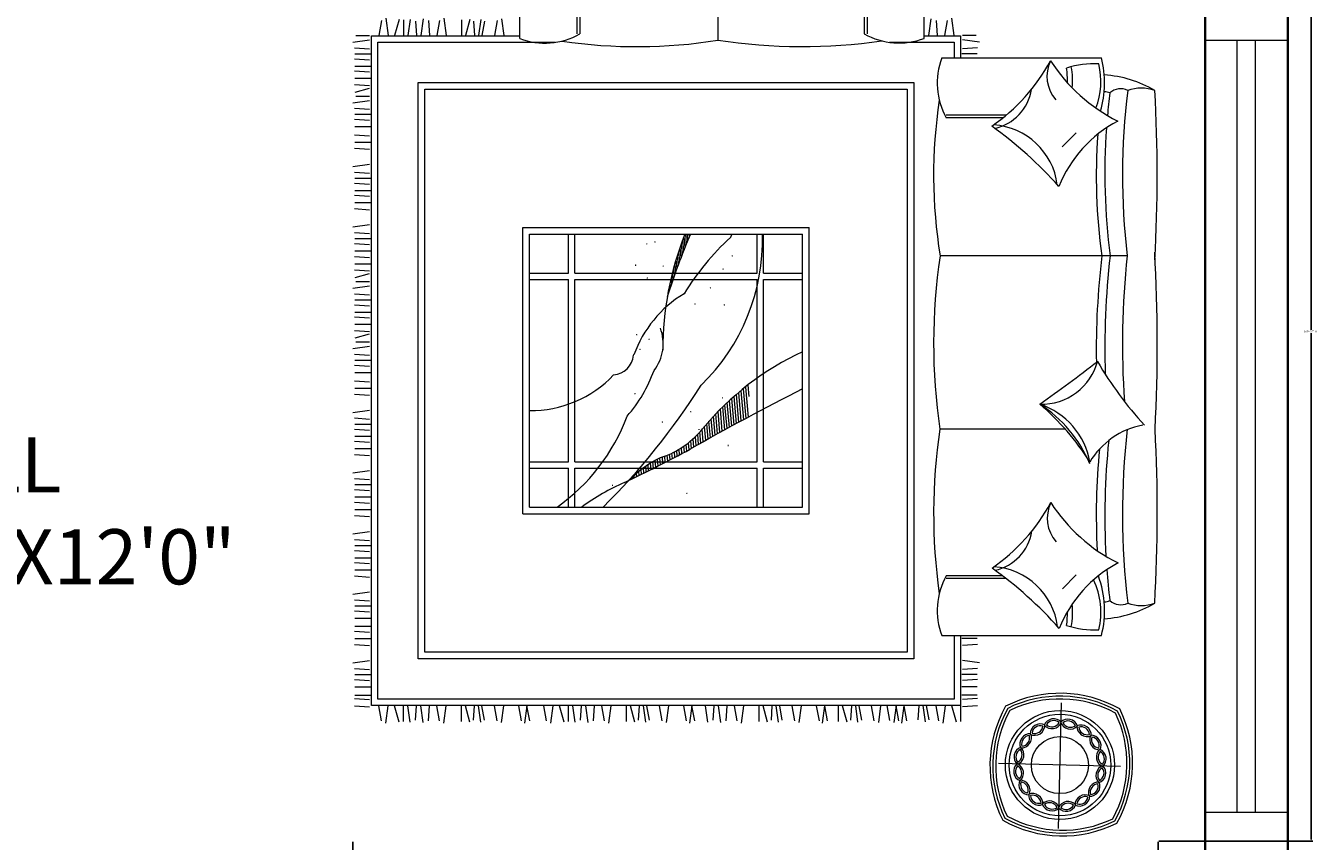
# Model space of a CAD drawing. Units: inches. Extents: x 1602 to 2642, y 1463 to 2270.
# Tile 3 of 5: x 1854 to 1995, y 1763 to 1851. Entities that reach past the tile are written whole.
import ezdxf

# ---------------------------------------------------------------- set-up
doc = ezdxf.new("R2010")
doc.units = ezdxf.units.IN
for name, color, linetype, lineweight in [('A-ANNO-DIMS', 2, 'Continuous', 18), ('A-AREA-IDEN', 7, 'Continuous', 18), ('A-FURN', 8, 'Continuous', 13), ('A-GLAZ', 4, 'Continuous', 18), ('A-WALL', 7, 'Continuous', 35)]:
    doc.layers.add(name, color=color, linetype=linetype, lineweight=lineweight)
doc.styles.get("Standard").update_dxf_attribs({"font": 'arial.ttf'})
doc.dimstyles.get("Standard").update_dxf_attribs({"dimtxt": 0.18, "dimasz": 0.18, "dimexe": 0.18, "dimexo": 0.0625, "dimgap": 0.09, "dimtad": 0, "dimtih": 1, "dimtoh": 1, "dimdec": 4, "dimzin": 0, "dimdsep": 46, "dimtxsty": 'Standard', "dimcen": 0.09, "dimadec": 0, "dimazin": 0, "dimtfac": 1, "dimtdec": 4, "dimtofl": 0, "dimtmove": 0, "dimatfit": 3, "dimfxl": 1, "dimtolj": 1, "dimtzin": 0, "dimarcsym": 0})

# ---------------------------------------------------------------- blocks, each defined once
blk = doc.blocks.new('A$C25EC1EFB')
h = blk.add_hatch()
h.set_pattern_fill('ANSI31', color=256, scale=2.508, angle=580, style=0)
h.set_pattern_definition([(94.99999999999984, (2801.512250582819, 4289.79602251789), (7.93259876143476, 0.6940124639253284), [])])
edge = h.paths.add_edge_path()
edge.add_ellipse((4084.490467177063, -2815.580363917667), major_axis=(-3872.16408689083, 3872.16408689083), ratio=0.9999999999995552, start_angle=340.89961915580596, end_angle=343.15488567038426, ccw=False)
edge.add_ellipse((1486.624568246823, 2293.159848771007), major_axis=(-194.6618757392838, 194.6618757392838), ratio=0.9999999999999246, start_angle=154.9056197196584, end_angle=183.4247301497222, ccw=False)
edge.add_ellipse((1687.117678346121, 1762.501521206774), major_axis=(-206.4950185728816, 206.4950185728816), ratio=0.999999999999898, start_angle=-23.5559095241906, end_angle=5.886608761987814)
edge.add_ellipse((823.8605303866296, 2467.162105106873), major_axis=(-581.4647167234576, 581.4647167234575), ratio=0.9999999999998493, start_angle=171.3363574034995, end_angle=185.7365630084011, ccw=False)
edge.add_line((1311.102457978037, 1804.744006331188), (1311.102457978037, 1908.515397835807))
edge.add_ellipse((-1407.416444189095, 7084.924681207201), major_axis=(4134.341428234145, 4134.341428234145), ratio=0.9999999999998351, start_angle=252.7073165240117, end_angle=254.8255249662156)
for p, q in [((317.5955949916479, 3231.219981357114), (307.6667150012017, 2827.177484563647)), ((117.9581545735291, 3031.926905659195), (509.944476949613, 3022.294292298837)), ((631.3901738150179, 2887.027849165279), (631.3901738150179, 2837.065101766894)), ((645.0795442243489, 2888.982161353262), (659.578070331745, 2837.065101766894)), ((688.1038474819233, 2892.890785729214), (680.5546081906668, 2837.065101766894)), ((701.7933985184081, 2885.073657987355), (710.5281339450539, 2837.065101766894)), ((732.7198837349368, 2882.204286455359), (741.09904921226, 2836.15004242288)), ((744.6795541957126, 2888.067102009248), (751.895255557758, 2836.15004242288)), ((767.9214057730514, 2882.204286455359), (764.7430494098026, 2836.15004242288)), ((804.5489009072134, 2885.073657987355), (813.2836363338665, 2837.065101766894)), ((820.5056566457297, 2892.890785729214), (812.9564173544732, 2837.065101766894)), ((830.489018271599, 2885.073657987355), (839.2237536982593, 2837.065101766894)), ((844.7281230778335, 2890.021414197218), (837.443163044978, 2836.15004242288)), ((858.8260332672307, 2884.158598643342), (867.5607686938984, 2836.15004242288)), ((894.9755861610774, 2890.936473541231), (887.690626128222, 2837.065101766894)), ((909.0734963504747, 2885.073657987355), (917.8082317771423, 2837.065101766894)), ((949.507840107568, 2883.119345799372), (957.8870055848911, 2837.065101766894)), ((961.4675105683438, 2888.982161353262), (968.683211930389, 2837.065101766894)), ((984.7093621456823, 2883.119345799372), (981.5310057824335, 2837.065101766894)), ((996.6690326064581, 2888.982161353262), (1011.167558713861, 2837.065101766894)), ((1023.822365107089, 2887.027849165279), (1023.822365107096, 2837.065101766894)), ((1059.561252837937, 2885.073657987355), (1068.29598826459, 2837.065101766894)), ((1075.518008576453, 2892.890785729214), (1067.968769285196, 2837.065101766894)), ((1085.501370202322, 2885.073657987355), (1094.236105628983, 2837.065101766894)), ((1149.987938091801, 2890.936473541231), (1142.702978058945, 2837.065101766894)), ((1164.085848281198, 2885.073657987355), (1172.820583707866, 2837.065101766894)), ((1204.520192038291, 2883.119345799372), (1212.899357515614, 2837.065101766894)), ((1216.479862499067, 2888.982161353262), (1223.695563861112, 2837.065101766894)), ((1239.721714076406, 2883.119345799372), (1236.543357713157, 2837.065101766894)), ((1251.681384537181, 2888.982161353262), (1266.179910644585, 2837.065101766894)), ((1278.834717037813, 2887.027849165279), (1278.83471703782, 2837.065101766894)), ((1335.548390704718, 2892.890785729214), (1327.999151413454, 2837.065101766894)), ((1349.237941741217, 2885.073657987355), (1357.972677167871, 2837.065101766894)), ((1384.439463779332, 2885.073657987355), (1381.126233840167, 2837.065101766894)), ((1402.040315111962, 2890.936473541231), (1409.52763688603, 2837.065101766894)), ((1426.2526619992, 2883.119345799372), (1423.074305635951, 2837.065101766894)), ((1443.853513331845, 2888.982161353262), (1451.069214693891, 2837.065101766894)), ((1485.909894853563, 2885.073657987355), (1494.644630280216, 2837.065101766894)), ((1501.866650592079, 2892.890785729214), (1494.317411300822, 2837.065101766894)), ((1511.850012217948, 2885.073657987355), (1520.584747644609, 2837.065101766894)), ((1576.336580107427, 2890.936473541231), (1569.051620074571, 2837.065101766894)), ((1590.434490296824, 2885.073657987355), (1599.169225723492, 2837.065101766894)), ((1630.868834053917, 2883.119345799372), (1639.247999531241, 2837.065101766894)), ((1642.828504514693, 2888.982161353262), (1650.044205876738, 2837.065101766894)), ((1666.070356092031, 2883.119345799372), (1662.891999728783, 2837.065101766894)), ((1678.030026552807, 2888.982161353262), (1692.528552660211, 2837.065101766894)), ((1705.183359053439, 2887.027849165279), (1705.183359053446, 2837.065101766894)), ((1761.897032720344, 2892.890785729214), (1754.34779342908, 2837.065101766894)), ((1775.586583756843, 2885.073657987355), (1784.321319183496, 2837.065101766894)), ((1810.788105794958, 2885.073657987355), (1807.474875855793, 2837.065101766894)), ((1828.388957127588, 2890.936473541231), (1835.876278901656, 2837.065101766894)), ((1852.601304014826, 2883.119345799372), (1849.422947651578, 2837.065101766894)), ((1870.202155347471, 2888.982161353262), (1877.417856709517, 2837.065101766894)), ((1891.714306976255, 2887.027849165279), (1891.714306976255, 2837.065101766894)), ((1905.403677385586, 2888.982161353262), (1919.902203492982, 2837.065101766894)), ((1948.427980643159, 2892.890785729214), (1940.878741351902, 2837.065101766894)), ((1962.117531679643, 2885.073657987355), (1970.852267106289, 2837.065101766894)), ((2015.857572578178, 2885.073657987355), (2024.592308004831, 2837.065101766894)), ((2031.814328316694, 2892.890785729214), (2024.265089025437, 2837.065101766894)), ((2041.797689942563, 2885.073657987355), (2050.532425369223, 2837.065101766894)), ((2106.284257832041, 2890.936473541231), (2098.999297799186, 2837.065101766894)), ((2120.382168021439, 2885.073657987355), (2129.116903448107, 2837.065101766894)), ((2160.816511778532, 2883.119345799372), (2169.195677255855, 2837.065101766894)), ((2172.776182239308, 2888.982161353262), (2179.991883601353, 2837.065101766894)), ((2196.018033816647, 2883.119345799372), (2192.839677453398, 2837.065101766894)), ((2207.977704277422, 2888.982161353262), (2222.476230384826, 2837.065101766894)), ((2235.131036778053, 2887.027849165279), (2235.131036778061, 2837.065101766894)), ((2291.844710444959, 2892.890785729214), (2284.295471153695, 2837.065101766894)), ((2305.534261481458, 2885.073657987355), (2314.268996908111, 2837.065101766894)), ((2340.735783519573, 2885.073657987355), (2337.422553580407, 2837.065101766894)), ((2358.336634852203, 2890.936473541231), (2365.823956626271, 2837.065101766894)), ((2382.548981739441, 2883.119345799372), (2379.370625376192, 2837.065101766894)), ((2400.149833072086, 2888.982161353262), (2407.365534434132, 2837.065101766894)), ((2421.66198470087, 2887.027849165279), (2421.66198470087, 2837.065101766894)), ((2435.351355110201, 2888.982161353262), (2449.849881217597, 2837.065101766894)), ((2478.375658367775, 2892.890785729214), (2470.826419076519, 2837.065101766894)), ((2492.06520940426, 2885.073657987355), (2500.799944830906, 2837.065101766894)), ((577.4890519529235, 2836.936244475415), (625.4976081733639, 2840.249474414588)), ((631.7592766263715, 2611.384835378944), (631.7592766263642, 2836.15004242288)), ((631.7592766263642, 2836.15004242288), (2524.304554552116, 2836.15004242288)), ((2524.304554552116, 2836.15004242288), (2524.304554552116, 684.1140680284224)), ((2578.574779225565, 2836.936244475415), (2530.566223005124, 2840.249474414588)), ((577.4890519529235, 2813.194849922737), (625.4976081733639, 2816.50807986191)), ((578.4283959861222, 2802.710657647047), (628.3911433845077, 2802.710657647047)), ((652.6592766263728, 2611.384835378944), (652.6592766263728, 2815.250042422886)), ((652.6592766263728, 2815.250042422886), (2503.404554552123, 2815.250042422886)), ((2503.404554552123, 2815.250042422886), (2503.404554552123, 705.0140680284312)), ((2577.635435192373, 2802.710657647047), (2527.672687793987, 2802.710657647047)), ((2578.574779225565, 2813.194849922737), (2530.566223005124, 2816.508079861895)), ((577.4890519529235, 2752.144911700663), (625.4976081733639, 2755.458141639836)), ((578.4283959861222, 2775.577635301154), (628.3911433845077, 2775.577635301154)), ((2577.635435192373, 2775.577635301154), (2527.672687793987, 2775.577635301154)), ((2578.574779225565, 2752.144911700663), (2530.566223005124, 2755.458141639836)), ((571.6262363990336, 2699.054774001932), (625.4976081733639, 2691.56745222785)), ((577.4890519529235, 2716.655625334541), (625.4976081733639, 2719.968855273714)), ((578.4283959861222, 2735.993497111231), (628.3911433845077, 2735.993497111231)), ((2577.635435192373, 2735.993497111231), (2527.672687793987, 2735.993497111231)), ((2578.574779225565, 2716.655625334541), (2530.566223005124, 2719.968855273714)), ((2584.437594779462, 2699.054774001932), (2530.566223005124, 2691.56745222785)), ((782.2392766263674, 834.5940680284328), (782.2392766263674, 2685.670042422884)), ((782.2392766263674, 2685.670042422884), (2373.824554552121, 2685.670042422884)), ((803.1392766263689, 855.4940680284271), (803.1392766263689, 2664.77004242289)), ((803.1392766263689, 2664.77004242289), (2352.924554552119, 2664.770042422875)), ((2352.924554552119, 2664.770042422875), (2352.924554552119, 855.4940680284271)), ((2373.824554552121, 2685.670042422884), (2373.824554552121, 834.5940680284328)), ((577.4890519529235, 2640.217478394574), (625.4976081733639, 2643.530708333732)), ((578.4283959861222, 2620.426176498651), (628.3911433845077, 2620.426176498651)), ((2577.635435192373, 2620.426176498651), (2527.672687793987, 2620.426176498651)), ((2578.574779225565, 2640.217478394574), (2530.566223005124, 2643.530708333732)), ((692.3034891433799, 2611.384835378944), (179.5334957905306, 2611.384835378958)), ((2577.635435192373, 2581.514517398078), (2527.672687793987, 2581.514517398078)), ((2578.574779225565, 2596.993452898176), (2530.566223005124, 2600.306682837334)), ((2577.635435192373, 2555.119914909323), (2527.672687793987, 2555.119914909323)), ((2578.574779225565, 2531.687191308833), (2530.566223005124, 2535.000421248005)), ((2577.635435192373, 2515.5357767194), (2527.672687793987, 2515.5357767194)), ((2578.574779225565, 2496.19790494271), (2530.566223005124, 2499.511134881883)), ((260.1263754639749, 2416.008756119314), (304.7479648114258, 2460.672138615999)), ((2584.437594779462, 2478.597053610102), (2530.566223005124, 2471.109731836019)), ((485.7932158359489, 2428.108270674471), (677.7791130337154, 2428.108270674471)), ((497.6695522999961, 2418.947027564289), (677.7791130337154, 2418.947027564289)), ((2578.574779225565, 2419.759758002729), (2530.566223005124, 2423.072987941902)), ((2577.635435192373, 2399.968456106821), (2527.672687793987, 2399.968456106821)), ((2578.574779225565, 2376.535732506331), (2530.566223005124, 2379.848962445518)), ((2577.635435192373, 2361.056797006248), (2527.672687793987, 2361.056797006248)), ((2578.574779225565, 2337.624073405757), (2530.566223005124, 2340.937303344916)), ((2577.635435192373, 2321.472658816325), (2527.672687793987, 2321.472658816325)), ((2578.574779225565, 2302.134787039635), (2530.566223005124, 2305.448016978807)), ((2584.437594779462, 2284.533935707012), (2530.566223005124, 2277.046613932944)), ((1118.231915589249, 2219.932055225661), (1118.231915589242, 1300.332055225655)), ((2037.831915589246, 2219.932055225647), (1118.231915589249, 2219.932055225661)), ((2037.831915589246, 2219.932055225647), (2037.831915589246, 1300.332055225655)), ((2577.635435192373, 2205.905338203745), (2527.672687793987, 2205.905338203745)), ((2578.574779225565, 2225.696640099654), (2530.566223005124, 2229.009870038812)), ((2016.931915589244, 2199.032055225638), (1139.131915589243, 2199.032055225638)), ((1139.131915589243, 2199.032055225638), (1139.131915589243, 1321.232055225664)), ((1264.531915589245, 2199.032055225638), (1264.531915589245, 2073.63205522563)), ((1285.431915589246, 2199.032055225638), (1285.431915589246, 2073.63205522563)), ((1870.631915589243, 2199.032055225638), (1870.631915589243, 2073.632055225644)), ((1891.531915589245, 2199.032055225638), (1891.531915589245, 2073.632055225644)), ((2016.931915589244, 2199.032055225638), (2016.931915589244, 1321.23205522565)), ((2577.635435192373, 2165.079528967945), (2527.672687793987, 2165.079528967945)), ((2578.574779225565, 2182.472614603256), (2530.566223005124, 2185.785844542428)), ((2577.635435192373, 2125.495390778036), (2527.672687793987, 2125.495390778036)), ((2578.574779225565, 2141.646805367455), (2530.566223005124, 2144.960035306627)), ((2578.574779225565, 2106.157519001346), (2530.566223005124, 2109.470748940505)), ((2584.437594779462, 2088.556667668723), (2530.566223005124, 2081.069345894641)), ((1264.531915589245, 2073.63205522563), (1139.131915589243, 2073.632055225644)), ((1264.531915589245, 2052.732055225635), (1139.131915589243, 2052.732055225664)), ((1264.531915589245, 2052.732055225635), (1264.531915589245, 1467.532055225652)), ((1870.631915589243, 2073.632055225644), (1285.431915589246, 2073.63205522563)), ((1870.631915589243, 2052.73205522565), (1285.431915589246, 2052.732055225635)), ((1285.431915589246, 2052.732055225635), (1285.431915589246, 1467.532055225652)), ((1870.631915589243, 2052.73205522565), (1870.631915589243, 1467.532055225652)), ((2016.931915589244, 2073.632055225658), (1891.531915589245, 2073.632055225644)), ((1891.531915589245, 2052.73205522565), (1891.531915589245, 1467.532055225652)), ((2016.931915589244, 2052.73205522565), (1891.531915589245, 2052.73205522565)), ((2577.635435192373, 2009.928070165443), (2527.672687793987, 2009.928070165443)), ((2578.574779225565, 2029.71937206135), (2530.566223005124, 2033.032602000523)), ((2577.635435192373, 1971.016411064869), (2527.672687793987, 1971.016411064869)), ((2578.574779225565, 1986.495346564967), (2530.566223005124, 1989.80857650414)), ((295.215244063229, 1948.444262769866), (698.1955948366831, 1948.444262769866)), ((2577.635435192373, 1931.432272874946), (2527.672687793987, 1931.432272874946)), ((2578.574779225565, 1947.583687464379), (2530.566223005124, 1950.896917403552)), ((2578.574779225565, 1912.094401098256), (2530.566223005124, 1915.407631037429)), ((2584.437594779454, 1894.493549765633), (2530.566223005124, 1887.006227991565)), ((2578.574779225565, 1835.656254158275), (2530.566223005124, 1838.969484097433)), ((2577.635435192373, 1815.864952262367), (2527.672687793987, 1815.864952262367)), ((2578.574779225565, 1792.432228661877), (2530.566223005124, 1795.74545860105)), ((2577.635435192373, 1765.828830553167), (2527.672687793987, 1765.828830553167)), ((2578.574779225565, 1742.396106952677), (2530.566223005124, 1745.70933689185)), ((2577.635435192373, 1726.244692363245), (2527.672687793987, 1726.244692363245)), ((2578.574779225565, 1706.906820586555), (2530.566223005124, 1710.220050525728)), ((2584.437594779454, 1689.305969253932), (2530.566223005124, 1681.818647479864)), ((2574.666154849634, 1667.793636998009), (2530.566223005124, 1667.793636998009)), ((2576.62046703761, 1655.01436679127), (2530.566223005124, 1642.153109532453)), ((2578.574779225565, 1630.468673646573), (2530.566223005124, 1633.781903585732)), ((2577.635435192373, 1610.677371750666), (2527.672687793987, 1610.677371750666)), ((2578.574779225565, 1587.244648150175), (2530.566223005124, 1590.557878089348)), ((2577.635435192373, 1571.765712650078), (2527.672687793987, 1571.765712650078)), ((2578.574779225565, 1548.332989049588), (2530.566223005124, 1551.646218988761)), ((1569.58961247749, 1498.845113355761), (1568.886649074042, 1506.88002182413)), ((1573.215999468995, 1518.30467450877), (1573.064505181503, 1520.03626213839)), ((2577.635435192373, 1532.18157446017), (2527.672687793987, 1532.18157446017)), ((2578.574779225565, 1512.84370268348), (2530.566223005124, 1516.156932622638)), ((2584.437594779454, 1495.242851350856), (2530.566223005124, 1487.755529576774)), ((1264.531915589245, 1467.532055225667), (1139.131915589243, 1467.532055225667)), ((1870.631915589243, 1467.532055225652), (1285.431915589246, 1467.532055225667)), ((1554.112776362645, 1432.108743085911), (1551.980974986758, 1456.475344311409)), ((1558.098049746682, 1447.466214001491), (1556.234828786708, 1468.762927025651)), ((1562.013830635669, 1463.617987770158), (1560.470927201475, 1481.253454721161)), ((1565.849127400865, 1480.689699283357), (1564.688483608976, 1493.955918529544)), ((2016.931915589244, 1467.532055225652), (1891.531915589245, 1467.532055225652)), ((2574.666154849634, 1473.730519094934), (2530.566223005124, 1473.730519094934)), ((2576.62046703761, 1460.951248888181), (2530.566223005124, 1448.089991629378)), ((1264.531915589245, 1446.632055225658), (1139.131915589243, 1446.632055225658)), ((1264.531915589245, 1446.632055225658), (1264.531915589245, 1321.23205522565)), ((1870.631915589243, 1446.632055225658), (1285.431915589246, 1446.632055225658)), ((1285.431915589246, 1446.632055225658), (1285.431915589246, 1321.23205522565)), ((1541.818491434993, 1389.905000426101), (1539.119938526573, 1420.749601311116)), ((1545.9666700701, 1403.400455801595), (1543.422872825396, 1432.476191356145)), ((1550.066663663807, 1417.446668720506), (1547.710096352946, 1444.382356338588)), ((1870.631915589243, 1446.632055225658), (1870.631915589243, 1321.23205522565)), ((1891.531915589245, 1446.632055225658), (1891.531915589245, 1321.23205522565)), ((2016.931915589244, 1446.632055225658), (1891.531915589245, 1446.632055225658)), ((2577.635435192373, 1416.61425384759), (2527.672687793987, 1416.61425384759)), ((2578.574779225565, 1436.405555743484), (2530.566223005124, 1439.718785682656)), ((96.56375242233663, 1391.350530609569), (178.0746753955263, 1391.350530609569)), ((178.0746753955263, 1391.350530609569), (697.7232225588759, 1391.350530609539)), ((1524.828260129872, 1340.466816335822), (1521.762395858635, 1375.50980530923)), ((1529.128590691436, 1352.223167233933), (1526.122610320157, 1386.58168009873)), ((1533.395763262031, 1364.358515703112), (1530.469269874078, 1397.808488191054)), ((1537.626860969483, 1376.906201744794), (1534.801885985626, 1409.195813564198)), ((2577.635435192373, 1374.823554733659), (2527.672687793987, 1374.823554733659)), ((2578.574779225565, 1393.181530247086), (2530.566223005124, 1396.494760186258)), ((1505.195571714308, 1321.23205522565), (1504.194793856486, 1332.670998484005)), ((1510.524449703889, 1321.232055225664), (1508.604887871583, 1343.172747367374)), ((1515.85332769347, 1321.232055225664), (1513.003113907138, 1353.810147877557)), ((1520.497301609701, 1329.060544606509), (1517.389086063931, 1364.587610862924)), ((2577.635435192373, 1335.239416543736), (2527.672687793987, 1335.239416543736)), ((2578.574779225565, 1351.390831133169), (2530.566223005124, 1354.704061072341)), ((2037.831915589246, 1300.332055225655), (1118.231915589242, 1300.332055225655)), ((2016.931915589244, 1321.23205522565), (1139.131915589243, 1321.232055225664)), ((1499.866693724727, 1321.232055225664), (1499.773196894175, 1322.300728889044)), ((2578.574779225565, 1315.901544767046), (2530.566223005124, 1319.214774706219)), ((2584.437594779454, 1298.300693434437), (2530.566223005124, 1290.81337166034)), ((2577.635435192373, 1219.672095931157), (2527.672687793987, 1219.672095931157)), ((2578.574779225565, 1239.463397827065), (2530.566223005124, 1242.776627766237)), ((2577.635435192373, 1180.760436830569), (2527.672687793987, 1180.760436830569)), ((2578.574779225565, 1196.239372330667), (2530.566223005124, 1199.552602269839)), ((2577.635435192373, 1141.176298640661), (2527.672687793987, 1141.176298640661)), ((2578.574779225565, 1157.327713230094), (2530.566223005124, 1160.640943169252)), ((2578.574779225565, 1121.838426863971), (2530.566223005124, 1125.151656803129)), ((2584.437594779454, 1104.237575531348), (2530.566223005124, 1096.75025375728)), ((261.0862426389085, 996.092857266216), (305.7078319863813, 1040.75623976293)), ((2578.574779225565, 1045.400279923975), (2530.566223005124, 1048.713509863148)), ((2577.635435192373, 1025.608978028081), (2527.672687793987, 1025.608978028081)), ((2578.574779225565, 1002.176254427577), (2530.566223005124, 1005.489484366764)), ((2577.635435192373, 975.5728563188677), (2527.672687793987, 975.5728563188677)), ((2578.574779225565, 952.1401327183776), (2530.566223005124, 955.4533626575503)), ((484.9045735572308, 938.6797065407083), (677.7791130337154, 938.6797065407083)), ((496.0354289729821, 947.8409496508756), (677.7791130337154, 947.8409496508756)), ((2577.635435192373, 935.9887181289595), (2527.672687793987, 935.9887181289595)), ((2578.574779225565, 916.6508463522696), (2530.566223005124, 919.9640762914278)), ((2584.437594779454, 899.0499950196463), (2530.566223005124, 891.5626732455638)), ((2574.666154849634, 877.5376627637233), (2530.566223005124, 877.5376627637233)), ((2373.824554552121, 834.5940680284328), (782.2392766263674, 834.5940680284328)), ((2352.924554552119, 855.4940680284271), (803.1392766263689, 855.4940680284271)), ((2576.62046703761, 864.7583925569852), (2530.566223005124, 851.8971352981679)), ((2578.574779225565, 840.2126994122737), (2530.566223005124, 843.5259293514464)), ((2577.635435192373, 820.4213975163657), (2527.672687793987, 820.4213975163657)), ((2578.574779225565, 796.9886739158756), (2530.566223005124, 800.3019038550628)), ((692.3034891433799, 755.403141836221), (179.5334957905306, 755.403141836221)), ((631.7592766263715, 684.1140680284224), (631.7592766263715, 755.4031418362065)), ((652.6592766263656, 705.0140680284312), (652.6592766263656, 755.403141836221)), ((2577.635435192373, 781.5097384157925), (2527.672687793987, 781.5097384157925)), ((2578.574779225565, 758.0770148153024), (2530.566223005124, 761.3902447544606)), ((577.4890519529235, 722.5877284491798), (625.4976081733639, 725.9009583883526)), ((578.4283959861222, 741.9256002258697), (628.3911433845077, 741.9256002258697)), ((2577.635435192373, 741.9256002258697), (2527.672687793987, 741.9256002258697)), ((2578.574779225565, 722.5877284491798), (2530.566223005124, 725.900958388338)), ((571.6262363990336, 704.9868771165566), (625.4976081733639, 697.4995553424742)), ((581.3976763288537, 683.4745448606335), (625.4976081733639, 683.4745448606335)), ((748.7809110632825, 684.1140680284224), (631.7592766263715, 684.1140680284224)), ((860.7261038871166, 705.0140680284312), (652.6592766263656, 705.0140680284312)), ((661.4278893405954, 627.3733247221026), (653.8786500493316, 683.1990086844235)), ((675.1174403770947, 635.1904524639612), (683.8521758037404, 683.1990086844235)), ((710.3189624152092, 635.1904524639612), (707.0057324760364, 683.1990086844235)), ((727.9198137478397, 629.3276369100713), (735.4071355219075, 683.1990086844235)), ((748.7809110632825, 692.29789009253), (748.7809110632752, 179.5278967396807)), ((932.0574757677549, 485.7876167851136), (932.0574757677622, 677.7735139828656)), ((941.2187188779444, 497.6639532491608), (941.2187188779517, 677.7735139828656)), ((1411.721483672338, 178.5414486224835), (1411.72148367236, 698.1899957858185)), ((1855.231064631016, 496.5022021999393), (1855.231064631016, 678.2458862606654)), ((1864.392307741191, 485.3713467841807), (1864.392307741191, 678.2458862606654)), ((2503.404554552123, 705.0140680284312), (1932.490745753996, 705.0140680284312)), ((2047.668872445676, 692.7702623703298), (2047.668872445669, 180.000269017466)), ((2524.304554552116, 684.1140680284224), (2047.668872445676, 684.1140680284224)), ((2106.284257832041, 629.3276369100713), (2098.999297799186, 683.1990086844235)), ((2120.382168021439, 635.1904524639612), (2129.116903448099, 683.1990086844235)), ((2160.816511778532, 637.1447646519445), (2169.195677255848, 683.1990086844235)), ((2172.776182239308, 631.2819490980546), (2179.991883601353, 683.1990086844235)), ((2196.018033816647, 637.1447646519445), (2192.839677453398, 683.1990086844235)), ((2207.977704277422, 631.2819490980546), (2222.476230384819, 683.1990086844235)), ((2235.131036778053, 633.2362612860233), (2235.131036778061, 683.1990086844235)), ((2291.844710444959, 627.3733247221026), (2284.295471153695, 683.1990086844235)), ((2305.534261481458, 635.1904524639612), (2314.268996908111, 683.1990086844235)), ((2340.735783519573, 635.1904524639612), (2337.422553580407, 683.1990086844235)), ((2358.336634852203, 629.3276369100713), (2365.823956626271, 683.1990086844235)), ((2382.548981739441, 637.1447646519445), (2379.370625376192, 683.1990086844235)), ((2400.149833072079, 631.2819490980546), (2407.365534434132, 683.1990086844235)), ((2421.66198470087, 633.2362612860233), (2421.66198470087, 683.1990086844235)), ((2435.351355110193, 631.2819490980546), (2449.849881217597, 683.1990086844235)), ((2478.375658367768, 627.3733247221026), (2470.826419076511, 683.1990086844235)), ((2492.065209404253, 635.1904524639612), (2500.799944830906, 683.1990086844235)), ((2584.437594779454, 704.9868771165566), (2530.566223005124, 697.4995553424742)), ((2574.666154849634, 683.4745448606335), (2530.566223005124, 683.4745448606335))]:
    blk.add_line(p, q)
at = {"const_width": 2.09}
for points in [[(1511.151005801041, 2155.427417849518, -1), (1511.151005801041, 2153.337417849522, -1)], [(1749.963977974703, 2129.419879811459, -1), (1749.963977974703, 2127.329879811463, -1)], [(1378.464403896922, 2001.982938292022, -1), (1378.464403896922, 1999.892938292025, -1)], [(1378.464403896922, 2000.937938292024, -1), (1378.464403896922, 1998.847938292026, -1)], [(1472.141222166467, 1950.101574691951, -1), (1472.141222166467, 1948.011574691955, -1)], [(1589.664228032883, 1926.272639169089, -1), (1589.664228032883, 1924.182639169077, -1)], [(1498.485842016862, 1893.112440112549, -1), (1498.485842016862, 1891.022440112552, -1)], [(1396.649697045645, 1848.538458734525, -1), (1396.649697045645, 1846.448458734528, -1)], [(1677.799055322533, 1835.246250902906, -1), (1677.799055322533, 1833.15625090291, -1)], [(1682.418605074026, 1710.698501999875, -1), (1682.418605074026, 1708.608501999864, -1)], [(1632.519993189891, 1660.01154033171, -1), (1632.519993189891, 1657.921540331714, -1)], [(1661.635412078192, 1692.493220240234, -1), (1661.635412078192, 1690.403220240223, -1)], [(1672.027005685611, 1645.679651771737, -1), (1672.027005685611, 1643.589651771741, -1)], [(1390.689109610934, 1549.797216376151, -1), (1390.689109610934, 1547.707216376155, -1)], [(1484.978268723158, 1546.850996961155, -1), (1484.978268723158, 1544.760996961158, -1)], [(1435.398901256181, 1495.038386561347, -1), (1435.398901256181, 1492.948386561351, -1)], [(1519.878047569999, 1513.762184183615, -1), (1519.878047569999, 1511.672184183619, -1)], [(1638.254319235255, 1463.626875239402, -1), (1638.254319235255, 1461.536875239391, -1)], [(1394.744337709578, 1434.839303017281, -1), (1394.744337709578, 1432.74930301727, -1)], [(1587.165183262217, 1425.04444594484, -1), (1587.165183262217, 1422.954445944844, -1)], [(1675.222175186443, 1421.779486743347, -1), (1675.222175186443, 1419.689486743351, -1)], [(1675.788258493603, 1422.657879986356, -1), (1675.788258493603, 1420.567879986345, -1)], [(1365.392005141164, 1392.394905260015, -1), (1365.392005141164, 1390.304905260018, -1)], [(1370.896625781812, 1333.067117625229, -1), (1370.896625781812, 1330.977117625232, -1)], [(1613.584636758898, 1347.361959619193, -1), (1613.584636758898, 1345.271959619196, -1)], [(1639.675595830262, 1353.891867756152, -1), (1639.675595830262, 1351.801867756156, -1)]]:
    blk.add_lwpolyline(points, format="xyb", close=True, dxfattribs=at)
for radius in [175.3148329503734, 163.2405281737082, 91.75760778478207, 91.75760778478207]:
    blk.add_circle((312.7783746963924, 3027.233248900499), radius)
for centre, radius, start, end in [((304.5060052362623, 2865.501903824778), 389.4856216215981, 60.51981844412023, 116.664792315698), ((304.5060052362623, 2865.501903824778), 380.3212540540306, 60.94048126723747, 116.2441294929664), ((468.7739130891368, 3021.890057497433), 389.4856216216183, 150.5198184440689, 206.6647923151855), ((468.7739130891368, 3021.890057497433), 380.3212540540507, 150.940481267197, 206.2441294932469), ((468.7739130891368, 3021.890057497433), 371.1568864864831, 151.3829579460627, 205.8016528138911), ((304.5060052362623, 2865.501903824778), 371.1568864864629, 61.3829579467198, 115.8016528138425), ((148.1178515636002, 3029.769811677652), 380.3212540540452, 330.940481267197, 26.24412949324692), ((148.1178515636002, 3029.769811677652), 389.4856216216128, 330.519818444069, 26.66479231518558), ((249.9997773948071, 3126.453250551473), 32.81996572270785, 64.15706611601946, 180.4877419729194), ((231.4874083348714, 3155.711586475598), 32.81996572270785, 244.1570661160195, 0.4877419729194889), ((292.7483643607866, 3142.924906735971), 32.81996572270785, 41.65706611607041, 157.9877419721565), ((286.8418459047189, 3177.040461384684), 32.81996572270785, 221.6570661160704, 337.9877419721565), ((292.7483643607866, 3142.924906735971), 27.09223599297813, 49.53860713232503, 150.106200956097), ((286.8418459047189, 3177.040461384684), 27.09223599297813, 229.5386071323251, 330.106200956097), ((338.5463388277367, 3141.783556762537), 32.81996572270785, 19.15706611564963, 135.4877419728042), ((346.1448848678137, 3175.562546198875), 32.81996572270785, 199.1570661156496, 315.4877419728042), ((338.5463388277367, 3141.783556762537), 27.09223599297813, 27.03860713130998, 127.6062009564518), ((346.1448848678137, 3175.562546198875), 27.09223599297813, 207.03860713131, 307.6062009564517), ((380.4213743429809, 3123.202960818256), 32.81996572270785, 356.6570661157543, 112.9877419724641), ((148.1178515636002, 3029.769811677652), 371.1568864864776, 331.3829579460627, 25.80165281389105), ((216.8086627786706, 3094.876248547203), 32.81996572270785, 86.65706611574215, 202.9877419731067), ((188.5087834891474, 3114.823049329724), 32.81996572270785, 266.6570661157422, 22.98774197310666), ((216.8086627786706, 3094.876248547203), 27.09223599297813, 94.53860713211645, 195.1062009565991), ((188.5087834891474, 3114.823049329724), 27.09223599297813, 274.5386071321164, 15.1062009565991), ((249.9997773948071, 3126.453250551473), 27.09223599297813, 72.03860713209241, 172.6062009563627), ((231.4874083348714, 3155.711586475598), 27.09223599297813, 252.0386071320924, 352.6062009563627), ((400.3681751255808, 3151.502840107795), 32.81996572270785, 176.6570661157543, 292.9877419724641), ((380.4213743429809, 3123.202960818256), 27.09223599297813, 4.538607132124711, 105.1062009564984), ((400.3681751255808, 3151.502840107795), 27.09223599297813, 184.5386071321247, 285.1062009564985), ((441.2567122714627, 3108.524215261983), 32.81996572270785, 154.1570661158802, 270.4877419729204), ((411.99837634733, 3090.011846202084), 32.81996572270785, 334.1570661158802, 90.48774197292038), ((441.2567122714627, 3108.524215261983), 27.09223599297813, 162.0386071315967, 262.6062009563761), ((411.99837634733, 3090.011846202084), 27.09223599297813, 342.0386071315967, 82.60620095637618), ((198.228066834361, 3053.001213031959), 32.81996572270785, 109.1570661156154, 225.4877419725107), ((198.228066834361, 3053.001213031959), 27.09223599297813, 117.0386071317286, 217.6062009569093), ((164.4490773980596, 3060.599759072014), 32.81996572270785, 289.1570661156154, 45.4877419725107), ((164.4490773980596, 3060.599759072014), 27.09223599297813, 297.0386071317287, 37.60620095690924), ((462.5855871805706, 3053.169777692201), 32.81996572270785, 131.6570661153347, 247.9877419725821), ((428.4700325318499, 3047.263259236141), 32.81996572270785, 311.6570661153347, 67.9877419725821), ((197.0867168608983, 3007.203238564958), 32.81996572270785, 131.6570661153347, 247.9877419725821), ((162.9711622121776, 3001.296720108883), 32.81996572270785, 311.6570661153347, 67.9877419725821), ((462.5855871805706, 3053.169777692201), 27.09223599297813, 139.5386071315111, 240.1062009565103), ((428.4700325318499, 3047.263259236141), 27.09223599297813, 319.5386071315111, 60.10620095651037), ((197.0867168608983, 3007.203238564958), 27.09223599297813, 139.5386071315111, 240.1062009565103), ((162.9711622121776, 3001.296720108883), 27.09223599297813, 319.5386071315111, 60.10620095651037), ((461.1076719946304, 2993.866738729142), 32.81996572270785, 109.1570661156154, 225.4877419725107), ((461.1076719946304, 2993.866738729142), 27.09223599297813, 117.0386071317286, 217.6062009569093), ((427.3286825583218, 3001.465284769183), 32.81996572270785, 289.1570661156154, 45.4877419725107), ((427.3286825583218, 3001.465284769183), 27.09223599297813, 297.0386071317287, 37.60620095690924), ((213.5583730454182, 2964.454651598957), 32.81996572270785, 154.1570661158802, 270.4877419729204), ((184.3000371212856, 2945.942282539014), 32.81996572270785, 334.1570661158802, 90.48774197292038), ((213.5583730454182, 2964.454651598957), 27.09223599297813, 162.0386071315967, 262.6062009563761), ((184.3000371212856, 2945.942282539014), 27.09223599297813, 342.0386071315967, 82.60620095637618), ((437.0479659035136, 2939.643448471507), 32.81996572270785, 86.65706611574215, 202.9877419731067), ((408.7480866139831, 2959.590249254084), 32.81996572270785, 266.6570661157422, 22.98774197310666), ((437.0479659035136, 2939.643448471507), 27.09223599297813, 94.53860713211645, 195.1062009565991), ((408.7480866139831, 2959.590249254084), 27.09223599297813, 274.5386071321164, 15.1062009565991), ((245.1353750497019, 2931.2635369829), 32.81996572270785, 176.6570661157543, 292.9877419724641), ((225.1885742671675, 2902.963657693362), 32.81996572270785, 356.6570661157543, 112.9877419724641), ((225.1885742671675, 2902.963657693362), 27.09223599297813, 4.538607132124711, 105.1062009564984), ((245.1353750497019, 2931.2635369829), 27.09223599297813, 184.5386071321247, 285.1062009564985), ((279.4118645249128, 2878.903951602297), 32.81996572270785, 19.15706611564963, 135.4877419728042), ((279.4118645249128, 2878.903951602297), 27.09223599297813, 27.03860713130998, 127.6062009564518), ((338.7149034880658, 2877.426036416531), 32.81996572270785, 41.65706611607041, 157.9877419721565), ((394.0693410578406, 2898.754911325472), 32.81996572270785, 64.15706611601946, 180.4877419729194), ((375.5569719979121, 2928.013247249612), 32.81996572270785, 244.1570661160195, 0.4877419729194889), ((394.0693410578406, 2898.754911325472), 27.09223599297813, 72.03860713209241, 172.6062009563627), ((375.5569719979121, 2928.013247249612), 27.09223599297813, 252.0386071320924, 352.6062009563627), ((287.0104105649825, 2912.682941038635), 32.81996572270785, 199.1570661156496, 315.4877419728042), ((287.0104105649825, 2912.682941038635), 27.09223599297813, 207.03860713131, 307.6062009564517), ((332.8083850320272, 2911.541591065259), 32.81996572270785, 221.6570661160704, 337.9877419721565), ((338.7149034880658, 2877.426036416531), 27.09223599297813, 49.53860713232503, 150.106200956097), ((332.8083850320272, 2911.541591065259), 27.09223599297813, 229.5386071323251, 330.106200956097), ((312.3857594164747, 3186.157965350322), 389.4856216216215, 240.5198184441202, 296.664792315698), ((312.3857594164747, 3186.157965350322), 380.321254054054, 240.9404812672375, 296.2441294929665), ((312.3857594164747, 3186.157965350322), 371.1568864864865, 241.3829579467198, 295.8016528138426), ((-66.97791102347219, 2741.235739154399), 411.4538102731095, 297.9946594870945, 338.1762138793086), ((485.6849424807896, 2530.614528687969), 316.6268320175827, 165.2207135339349, 200.5803261067808), ((418.6501303724453, 2535.610501958414), 237.4397884308417, 166.1700435477292, 205.7780897744892), ((204.339334419632, 2318.693444448676), 274.1566884687789, 71.51504750021564, 93.39711909964328), ((497.8312535542154, 2538.16598036026), 225.8008880027097, 168.6738781631475, 187.0247756611673), ((598.0274163895828, 2538.727136571623), 309.3592482736565, 172.5749152310043, 180.8047485918571), ((1283.508809838853, 3449.962053271382), 1296.354628148881, 221.6592367374925, 234.5116366288277), ((540.2630908703158, 2611.491247017526), 221.9945356540506, 187.5079417690746, 265.9655471801888), ((480.3582111107698, 2530.614528687969), 226.8141162345917, 330.5061277685731, 20.86136247484521), ((195.6843466176888, 2185.033945401934), 372.842184662441, 93.92554538864677, 120.1803651628055), ((4996.65887399418, 2220.360220203446), 4996.658984712837, 176.7074856531786, 183.1195518594664), ((51.72331663881232, 2379.511204224975), 135.0162301971975, 71.21591897210322, 108.7840810278968), ((117.6290057528549, 2460.596579721278), 51.84314058293741, 47.65613945501247, 115.6360597975105), ((-2360.09590959807, 2220.36177111102), 2472.008696990425, 353.6847648439718, 6.66647620846205), ((170.0372764724398, 2463.430468606363), 39.55947945866067, 89.66938794367344, 116.2356847377325), ((-2188.900113372524, 2225.452933450542), 2357.364478536592, 4.231825415872696, 6.661489045370558), ((-1103.410099498576, 2219.652800483375), 1821.904813317624, 351.4391390897871, 8.07806386477066), ((-122.8084356441159, 1883.397110391328), 553.6612235346786, 32.89311831868918, 63.27775504761099), ((872.4576201586259, 1897.897328879502), 602.6484764389724, 124.5216399525099, 151.6492334142083), ((554.2118058471041, 2252.446735564743), 152.68412196255, 102.5229511726573, 171.0221639720541), ((-2188.900113372524, 2225.452933450542), 2357.364478536592, 354.1380716214208, 3.186339755773678), ((-1934.092949295291, 2222.16245300974), 2130.205316173485, 354.3366119699191, 3.122340433890637), ((236.6502300063749, 2234.140918228608), 116.724496395002, 334.6012084837302, 40.54519748807014), ((3333.68451552435, 627.3607967675852), 2209.54164879086, 134.6725360764692, 147.7436105193565), ((2287.848786312694, 1688.392912899486), 624.2670274309789, 125.1781643370384, 159.5766212149076), ((1462.653166443046, 2709.567626046374), 640.2705249755662, 292.8904712152515, 307.0626715443762), ((4084.490467176721, -2815.580363917798), 5476.066967415318, 115.6772969660199, 118.1548856704495), ((1486.624568246801, 2293.159848771022), 275.2934647474958, 289.9056197197872, 318.4247301496573), ((-0.6177152241562, 2184.48465062114), 253.9477150983728, 280.7511909839713, 329.0494423525057), ((453.6099681309151, 2096.170622020225), 240.7975200416083, 190.0700186547298, 251.513634063623), ((908.7840328066176, 2490.587393829039), 818.7709283277208, 212.2985283174918, 229.5205449398777), ((605.8689457633682, 2221.784951912334), 421.389769092894, 202.7175797507866, 237.1449020849582), ((1687.117678346143, 1762.501521206774), 292.0280558282651, 111.4440904757719, 140.8866087620124), ((-2476.242387987366, 8989.86383017015), 8031.077363206627, 296.7547849003873, 299.6814985470403), ((5189.150422587271, 1671.336334253319), 5189.15053347117, 176.9388687943686, 183.2308528880728), ((-839.4520402920297, 1128.346231058596), 1194.536584156627, 30.28757816154475, 42.47600852879704), ((-1180.980868497192, 1671.490592317997), 1899.475589715449, 351.5189182688073, 8.383916999333405), ((751.7750952702208, 2534.062472635524), 920.4881034674244, 294.8861636343854, 320.3521788954757), ((2051.740526511305, 1602.642054351665), 462.5051862275705, 138.9735804164881, 160.2295429731453), ((2014.166362558564, 1518.116840648719), 370.3125627779616, 89.60713639418466, 136.3509345096815), ((-2542.961442119571, 1676.420809756869), 2654.874444615911, 353.8359141254732, 3.941589238157162), ((371.9425472902603, 1681.276073594003), 186.5981164301189, 88.3676044124178, 165.4240521520288), ((6758.791727714807, -6953.703300457077), 10887.73917538406, 125.8822296803705, 127.0946183806769), ((1916.655318256047, 1341.313739382756), 648.3552410927683, 134.1383379809644, 181.6847040310653), ((-2506.397899627386, 1689.565239908428), 2674.862814158767, 353.5989091821728, 1.753625510809246), ((1726.67177394053, 1673.301525916809), 139.6326613666137, 142.0948538523169, 200.8895128689712), ((1752.222980010354, 1704.369846744921), 69.61106324809847, 94.95105755802923, 174.8766543317414), ((-2326.042400942924, 1692.457594399231), 2522.155386940687, 353.1433999362063, 0.9352784211903266), ((1322.831429736014, 1838.987718223034), 381.1559142689087, 301.1293017828129, 340.1644872338225), ((576.7142338831854, 1693.940106953196), 1011.861440092256, 338.386783207812, 0.0010917430398909), ((792.9020607460498, 1960.337764563381), 853.7319657820956, 312.6112985239825, 328.3781661717325), ((-408.4163850434979, 2142.027900565321), 2076.810081976653, 336.7203354898851, 342.6666348099279), ((4495.264646208692, 1131.636235892503), 4495.264757303411, 176.5286646489921, 183.4713353510079), ((-2103.057569686191, 1131.043567661028), 2214.970355475213, 352.9568681005381, 6.749091233589736), ((-1942.059593270771, 1126.570840005042), 2110.523956920629, 356.0103517824921, 7.207139134266308), ((-1679.127574485506, 1131.881667123445), 1875.239794821453, 355.979905590025, 7.953287269012241), ((-903.4661616481953, 1132.604370050168), 1621.960856402422, 351.4376268635095, 9.179428766552546), ((1307.752931048004, 1350.181809599417), 65.70312471435534, 333.8568999860387, 343.9551289370007), ((-66.01804384855313, 1321.319840301301), 411.4538102731095, 297.9946594870945, 338.1762138793086), ((1284.468677013779, 2030.046154418269), 1296.354628148881, 221.6592367374925, 234.5116366288277), ((541.2229580452349, 1191.575348164413), 221.9945356540506, 187.5079417690746, 265.9655471801888), ((-121.8485684691895, 463.4812115382446), 553.6612235346786, 32.89311831868918, 63.27775504761099), ((873.4174873335451, 477.9814300264042), 602.6484764389724, 124.5216399525099, 151.6492334142083), ((555.1716730220232, 832.5308367116448), 152.68412196255, 102.5229511726573, 171.0221639720541), ((-1942.059593270771, 1126.570840005042), 2110.523956920629, 352.959262168444, 354.9261967154591), ((485.6849424807824, 836.1734485271663), 316.6268320175827, 163.4758498436011, 194.7792864660651), ((418.650130372438, 831.1774752567508), 237.4397884308417, 159.0286918999472, 193.8299564522708), ((480.3582111107625, 836.1734485271663), 226.8141162345917, 339.1386375251548, 29.49387223142695), ((237.6100971813012, 814.2250193755099), 116.724496395002, 334.6012084837302, 40.54519748807014), ((51.72331663881232, 987.2767729902044), 135.0162301971975, 251.2159189721032, 288.7840810278968), ((195.6843466176888, 1181.754031813245), 372.842184662441, 239.8196348371945, 266.0744546113532), ((117.6290057528549, 906.191397493887), 51.84314058293741, 244.3639402024895, 312.3438605449875), ((170.0372764724325, 903.3575086087877), 39.55947945866067, 243.7643152622675, 270.3306120563266), ((497.8312535542154, 828.6219968549048), 225.8008880027097, 174.2072358022055, 191.3261218368525), ((598.0274163895756, 828.0608406435421), 309.3592482736565, 178.732558296228, 187.4250847689957), ((204.339334419632, 1048.094532766488), 274.1566884687789, 266.6028809003567, 288.4849524997843), ((829.5512177542569, 480.3526120599344), 226.8141162345917, 60.50612776871507, 110.8613624749055), ((1140.512945958866, -1103.415698549412), 1821.904813317624, 81.43913909021488, 98.07806386468211), ((1670.467644231738, -902.9993884212234), 1621.960856402422, 81.43762686347846, 99.17942876656917), ((1966.898565754723, 480.8249843377198), 226.8141162345917, 69.13863752509452, 119.4938722312849)]:
    blk.add_arc(centre, radius, start, end)
blk = doc.blocks.new('WIN-84IN')
for p, q in [((2.274e-13, 83.99999999999977), (8.999999999999773, 83.99999999999977)), ((3.5, -2.274e-13), (3.5, 84)), ((5.5, -2.274e-13), (5.5, 84)), ((2.274e-13, -2.274e-13), (8.999999999999773, -2.274e-13))]:
    blk.add_line(p, q)
blk = doc.blocks.new('*D19')
at = {"layer": 'A-ANNO-DIMS', "color": 0, "lineweight": -2, "transparency": 16777216}
for p, q in [((1977.681887442998, 1873.678767726278), (1994.435915796376, 1873.678767726278)), ((1994.255915796377, 1873.498767726278), (1994.255915796377, 1818.406804183643)), ((1994.255915796377, 1762.948578703764), (1994.255915796377, 1818.040542246398)), ((1977.681887442998, 1762.768578703764), (1994.435915796376, 1762.768578703764))]:
    blk.add_line(p, q, dxfattribs=at)
at = {"layer": 'A-ANNO-DIMS', "color": 0, "transparency": 16777216}
for points in [[(1994.225915796377, 1873.498767726278), (1994.285915796377, 1873.498767726278), (1994.255915796377, 1873.678767726278)], [(1994.225915796377, 1762.948578703764), (1994.285915796377, 1762.948578703764), (1994.255915796377, 1762.768578703764)]]:
    blk.add_solid(points, dxfattribs=at)
at = {"layer": 'Defpoints', "color": 0, "transparency": 16777216}
for p in [(1977.619387442998, 1873.678767726278), (1977.619387442998, 1762.768578703764), (1994.255915796377, 1762.768578703764)]:
    blk.add_point(p, dxfattribs=at)
at = {"layer": 'A-ANNO-DIMS', "color": 0, "transparency": 16777216, "insert": (1994.255915796377, 1818.22367321502), "char_height": 0.18, "attachment_point": 5}
blk.add_mtext('\\A1;SOFA SET 111', dxfattribs=at)
blk = doc.blocks.new('*D20')
at = {"layer": 'A-ANNO-DIMS', "color": 0, "lineweight": -2, "transparency": 16777216}
for p, q in [((1889.991112678977, 1762.706078703763), (1889.991112678977, 1745.952050350386)), ((1977.619387442997, 1762.706078703763), (1977.619387442997, 1745.952050350386)), ((1890.171112678977, 1746.132050350386), (1933.586020865898, 1746.132050350386)), ((1977.439387442997, 1746.132050350386), (1934.024479256076, 1746.132050350386))]:
    blk.add_line(p, q, dxfattribs=at)
at = {"layer": 'A-ANNO-DIMS', "color": 0, "transparency": 16777216}
for points in [[(1890.171112678977, 1746.162050350386), (1890.171112678977, 1746.102050350386), (1889.991112678977, 1746.132050350386)], [(1977.439387442997, 1746.162050350386), (1977.439387442997, 1746.102050350386), (1977.619387442997, 1746.132050350386)]]:
    blk.add_solid(points, dxfattribs=at)
at = {"layer": 'Defpoints', "color": 0, "transparency": 16777216}
for p in [(1889.991112678977, 1762.768578703763), (1977.619387442997, 1762.768578703763), (1889.991112678977, 1746.132050350386)]:
    blk.add_point(p, dxfattribs=at)
at = {"layer": 'A-ANNO-DIMS', "color": 0, "transparency": 16777216, "insert": (1933.805250060987, 1746.132050350386), "char_height": 0.18, "attachment_point": 5}
blk.add_mtext('\\A1;88', dxfattribs=at)

msp = doc.modelspace()

# ---------------------------------------------------------------- linework, layer by layer
at = {"layer": 'A-WALL'}
for p, q in [((1991.726933683589, 2040.248102623293), (1991.726933683589, 1725.248102623292)), ((1982.726933683589, 1878.248102623292), (1982.726933683589, 1725.248102623293))]:
    msp.add_line(p, q, dxfattribs=at)

# ---------------------------------------------------------------- block references
at = {"layer": 'A-FURN', "xscale": 0.0338700972235775, "yscale": 0.0338700972235775, "zscale": 0.0338700972235775, "rotation": 180}
msp.add_blockref('A$C25EC1EFB', (1977.526265282426, 1873.585705524922), dxfattribs=at)
at = {"layer": 'A-GLAZ'}
msp.add_blockref('WIN-84IN', (1982.726933683589, 1765.938566686288), dxfattribs=at)

# ---------------------------------------------------------------- texts
at = {"layer": 'A-AREA-IDEN', "insert": (1832.997583607896, 1806.717258268221), "char_height": 6, "attachment_point": 1}
msp.add_mtext_dynamic_manual_height_columns('   HALL\\P19\'3"X12\'0"', width=62.85526611132081, gutter_width=12.5, heights=[0], dxfattribs=at)

# ---------------------------------------------------------------- dimensions: what is measured, and where the dimension line sits
at = {"layer": 'A-ANNO-DIMS'}
dim = msp.add_linear_dim(base=(1994.255915796377, 1762.768578703764), p1=(1977.619387442997, 1873.678767726277), p2=(1977.619387442997, 1762.768578703763), angle=270, text='SOFA SET <>', dimstyle='Standard', override={"dimdec": 0, "dimlfac": 1, "dimrnd": 0, "dimzin": 0, "dimdsep": 46, "dimlunit": 2}, dxfattribs=at)
dim.commit()
dim.dimension.update_dxf_attribs({"geometry": '*D19', "text_midpoint": (1994.255915796377, 1818.22367321502)})
dim = msp.add_linear_dim(base=(1889.991112678977, 1746.132050350386), p1=(1977.619387442997, 1762.768578703763), p2=(1889.991112678977, 1762.768578703763), angle=180, dimstyle='Standard', override={"dimdec": 0, "dimlfac": 1, "dimrnd": 0, "dimzin": 0, "dimdsep": 46, "dimlunit": 2}, dxfattribs=at)
dim.commit()
dim.dimension.update_dxf_attribs({"geometry": '*D20', "text_midpoint": (1933.805250060987, 1746.132050350386)})

doc.saveas('drawing.dxf')
